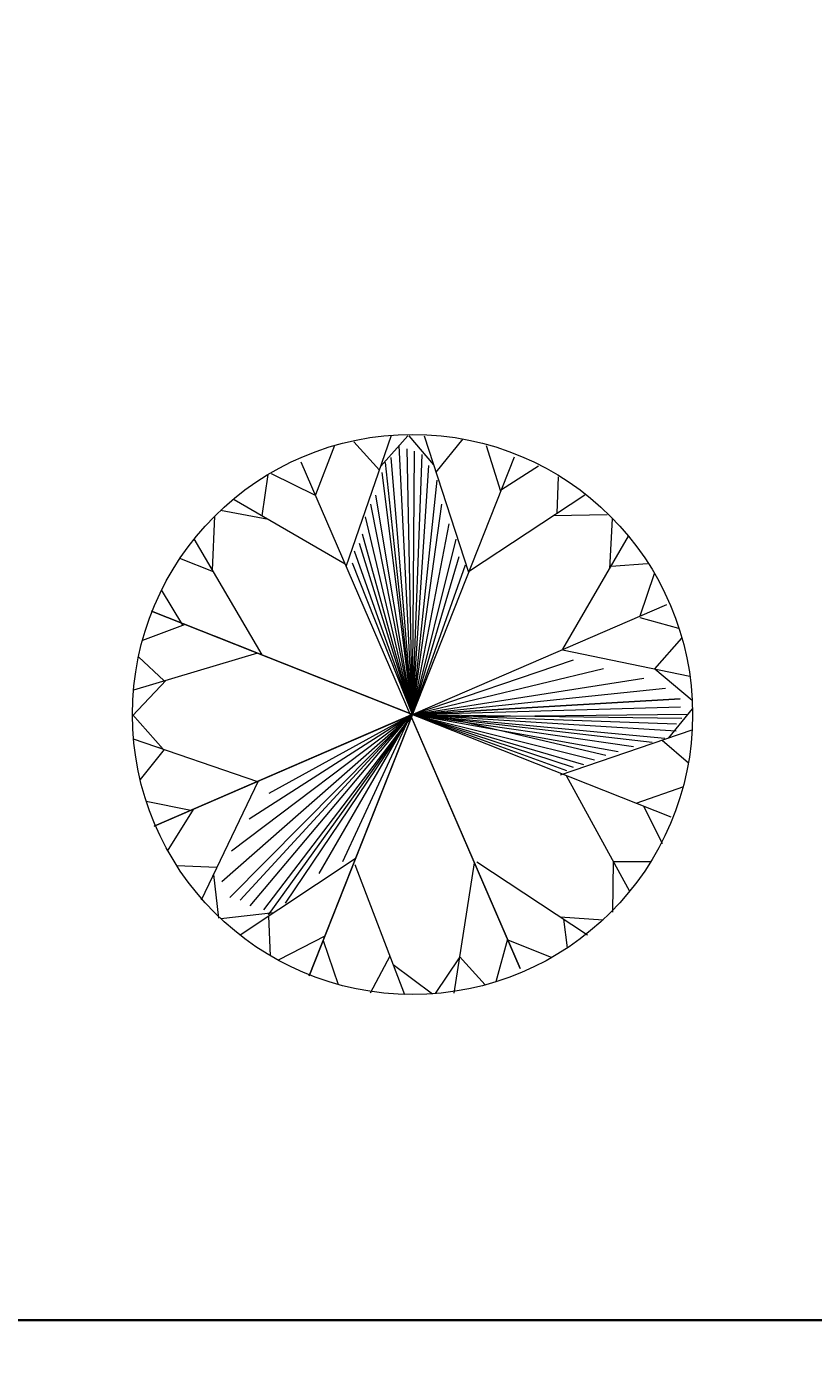
# Model space of a CAD drawing. Units: inches. Extents: x 8049 to 8459, y 820 to 1350.
# Tile 10 of 25: x 8157 to 8170, y 853 to 877. Entities that reach past the tile are written whole.
import ezdxf

# ---------------------------------------------------------------- set-up
doc = ezdxf.new("R2010")
doc.units = ezdxf.units.IN
doc.header["$MEASUREMENT"] = 0
for name, color, linetype, lineweight in [('A-ANNO-DIMS', 2, 'Continuous', 18), ('C-SITE-WALL', 7, 'Continuous', 35), ('zelen', 69, 'Continuous', 13)]:
    doc.layers.add(name, color=color, linetype=linetype, lineweight=lineweight)
doc.styles.get("Standard").update_dxf_attribs({"font": 'arial.ttf'})
doc.dimstyles.get("Standard").update_dxf_attribs({"dimtxt": 0.18, "dimasz": 0.18, "dimexe": 0.18, "dimexo": 0.0625, "dimgap": 0.09, "dimtad": 0, "dimtih": 1, "dimtoh": 1, "dimdec": 4, "dimzin": 0, "dimdsep": 46, "dimtxsty": 'Standard', "dimcen": 0.09, "dimadec": 0, "dimazin": 0, "dimtfac": 1, "dimtdec": 4, "dimtofl": 0, "dimtmove": 0, "dimatfit": 3, "dimfxl": 1, "dimtolj": 1, "dimtzin": 0, "dimarcsym": 0})

# ---------------------------------------------------------------- blocks, each defined once
blk = doc.blocks.new('T40C')
for p, q in [((-0.1219, 0.4263), (-0.1133, 0.5002)), ((-0.0016, 0.4444), (-0.055, 0.5069)), ((-0.0016, 0.0138), (-0.0016, 0.5115)), ((-0.0016, 0.5115), (-0.0016, -0.4769)), ((-0.0016, 0.4364), (0.0585, 0.5048)), ((0.1041, 0.4402), (0.0754, 0.5038)), ((-0.0047, 0.2984), (-0.1711, 0.4799)), ((-0.0016, 0.2889), (0.1386, 0.4896)), ((0.2217, 0.4068), (0.1848, 0.4759)), ((-0.2374, 0.3843), (-0.221, 0.4586)), ((-0.1327, 0.438), (-0.2166, 0.4607)), ((0.0979, 0.4313), (0.1806, 0.4751)), ((0.2091, 0.2244), (0.2252, 0.4573)), ((-0.2, 0.2178), (-0.2513, 0.4459)), ((-0.0016, 0.0138), (0.1054, 0.4378)), ((-0.0016, 0.0138), (0.1166, 0.4328)), ((0.0011, 0.0164), (0.1417, 0.4349)), ((0.0011, 0.0164), (0.1801, 0.4343)), ((0.0011, 0.0164), (0.161, 0.432)), ((-0.2369, 0.3817), (-0.2976, 0.4118)), ((-0.0016, 0.0138), (0.2033, 0.4135)), ((-0.0016, 0.0138), (0.0852, 0.4075)), ((0.2208, 0.3933), (0.2879, 0.4166)), ((-0.3045, 0.3219), (-0.313, 0.3998)), ((0.2979, 0.3132), (0.3134, 0.399)), ((0.3508, 0.3661), (-0.3487, -0.3333)), ((0.0011, 0.0164), (-0.3443, 0.3618)), ((-0.3443, 0.3618), (0.3464, -0.329)), ((-0.0016, 0.0138), (0.2072, 0.3567)), ((0.0011, 0.0164), (0.3508, 0.3661)), ((0.0011, 0.0164), (0.0491, 0.3369)), ((-0.3055, 0.3229), (-0.3893, 0.3231)), ((0.3008, 0.3162), (0.3801, 0.3306)), ((-0.3838, 0.2523), (-0.4084, 0.2975)), ((-0.0016, 0.0138), (0.1989, 0.2926)), ((0.0011, 0.0164), (0.0175, 0.3021)), ((0.3847, 0.2335), (0.4047, 0.2984)), ((-0.2034, 0.2144), (-0.4335, 0.2627)), ((-0.377, 0.2509), (-0.4492, 0.2275)), ((-0.0016, 0.0138), (0.1836, 0.2378)), ((0.2092, 0.2254), (0.4418, 0.2362)), ((0.3861, 0.2336), (0.4597, 0.1963)), ((0.3915, 0.2339), (0.3982, 0.2342)), ((-0.4278, 0.1246), (-0.4601, 0.209)), ((0.4263, 0.1181), (0.4586, 0.1989)), ((-0.2946, 0.0138), (-0.4744, 0.1635)), ((0.2937, 0.0138), (0.4738, 0.1555)), ((-0.4281, 0.1249), (-0.4899, 0.1006)), ((0.4291, 0.1204), (0.4873, 0.0978)), ((-0.4418, 0.0138), (-0.4967, 0.0634)), ((0.4315, 0.0138), (0.491, 0.0679)), ((-0.4277, 0.0138), (-0.4952, -0.0443)), ((0.4953, 0.0138), (-0.4939, 0.0138)), ((-0.2846, 0.0167), (-0.4721, -0.1432)), ((-0.0016, 0.0138), (-0.4477, -0.1559)), ((-0.0016, 0.0138), (-0.4464, -0.1312)), ((-0.0016, 0.0138), (-0.4422, -0.1429)), ((-0.0016, 0.0138), (-0.4379, -0.1735)), ((-0.0016, 0.0138), (-0.4328, -0.1117)), ((-0.0016, 0.0138), (-0.4324, -0.1862)), ((-0.4324, -0.1862), (-0.0016, 0.0138)), ((-0.0016, 0.0138), (-0.4146, -0.0968)), ((-0.0016, 0.0138), (-0.4013, -0.1946)), ((-0.0016, 0.0138), (-0.3864, -0.0775)), ((-0.0016, 0.0138), (-0.3647, -0.0593)), ((-0.0016, 0.0138), (-0.3588, -0.1967)), ((-0.0016, 0.0138), (-0.3309, -0.0302)), ((-0.0016, 0.0138), (-0.3156, -0.0151)), ((-0.0016, 0.0138), (-0.3007, -0.0042)), ((-0.0016, 0.0138), (-0.2917, 0.0059)), ((-0.0016, 0.0138), (-0.2861, -0.1863)), ((-0.0016, 0.0138), (-0.2311, -0.181)), ((-0.0016, 0.0138), (-0.0528, -0.0021)), ((-0.0016, 0.0138), (-0.0528, -0.0021)), ((-0.0016, 0.0138), (0.0011, 0.0164)), ((-0.0016, 0.0138), (0.4953, 0.0138)), ((-0.0016, 0.0138), (0.0088, -0.2669)), ((-0.0016, 0.0138), (0.0243, -0.2768)), ((-0.0016, 0.0138), (0.0408, -0.3033)), ((-0.0016, 0.0138), (0.0625, -0.3241)), ((-0.0016, 0.0138), (0.0872, -0.3518)), ((-0.0016, 0.0138), (0.1104, -0.3878)), ((-0.0016, 0.0138), (0.1339, -0.4064)), ((-0.0016, 0.0138), (0.1521, -0.4202)), ((-0.0016, 0.0138), (0.1669, -0.4211)), ((-0.0016, 0.0138), (0.1801, -0.4202)), ((-0.0016, 0.0138), (0.1959, -0.4202)), ((-0.0016, 0.0138), (0.2013, -0.3955)), ((-0.0016, 0.0138), (0.2072, -0.3832)), ((-0.0016, 0.0138), (0.2062, -0.3647)), ((-0.0016, 0.0138), (0.2018, -0.3233)), ((-0.0016, 0.0138), (0.2038, -0.3052)), ((-0.0016, 0.0138), (0.2044, -0.2809)), ((-0.0016, 0.0138), (0.1983, -0.2504)), ((-0.0016, 0.0138), (0.197, -0.2334)), ((-0.0016, 0.0138), (0.2007, -0.2173)), ((-0.0016, 0.0138), (0.1959, -0.1959)), ((0.285, 0.0138), (0.4722, -0.133)), ((0.2917, 0.0138), (0.3747, 0.0138)), ((0.4349, 0.0169), (0.4927, -0.0276)), ((-0.0528, -0.0021), (-0.4551, -0.1664)), ((-0.0528, -0.0021), (-0.3463, -0.045)), ((-0.4294, -0.1068), (-0.4874, -0.0863)), ((0.4191, -0.0914), (0.4833, -0.0909)), ((0.4217, -0.0934), (0.4533, -0.184)), ((-0.4387, -0.1147), (-0.459, -0.1779)), ((0.2042, -0.1867), (0.2149, -0.4325)), ((0.2071, -0.1897), (0.4318, -0.2236)), ((-0.3712, -0.2192), (-0.4529, -0.1923)), ((-0.2066, -0.1906), (-0.4335, -0.23)), ((-0.2067, -0.1914), (-0.2414, -0.4204)), ((0.3628, -0.2132), (0.4476, -0.1967)), ((-0.3712, -0.2192), (-0.3953, -0.2872)), ((0.3755, -0.2151), (0.3928, -0.2871)), ((-0.0016, -0.2596), (-0.1424, -0.4599)), ((-0.0016, -0.2565), (0.16, -0.4525)), ((0.3007, -0.2833), (0.3874, -0.2905)), ((0.3008, -0.2851), (0.3017, -0.3787)), ((-0.3126, -0.2938), (-0.3837, -0.3016)), ((-0.3124, -0.2971), (-0.3082, -0.3761)), ((-0.2315, -0.3548), (-0.2033, -0.4394)), ((-0.2322, -0.3601), (-0.2902, -0.3882)), ((0.2123, -0.3741), (0.1875, -0.442)), ((0.212, -0.3667), (0.2724, -0.3967)), ((0.1172, -0.4006), (0.0947, -0.4728)), ((-0.1046, -0.4061), (-0.1917, -0.4425)), ((-0.1086, -0.4118), (-0.0869, -0.4727)), ((-0.0016, -0.4144), (-0.047, -0.4779)), ((-0.0016, -0.4109), (0.0515, -0.477)), ((0.1259, -0.4112), (0.1857, -0.4428))]:
    blk.add_line(p, q)
blk.add_circle((-0.0016, 0.0138), 0.496)
blk = doc.blocks.new('*D58')
at = {"layer": 'A-ANNO-DIMS', "color": 0, "lineweight": -2, "transparency": 16777216}
for p, q in [((8139.397, 1162.808), (8139.397, 820.091)), ((8175.397, 1162.808), (8175.397, 820.091)), ((8139.577, 820.271), (8157.179, 820.271)), ((8175.217, 820.271), (8157.616, 820.271))]:
    blk.add_line(p, q, dxfattribs=at)
at = {"layer": 'A-ANNO-DIMS', "color": 0, "transparency": 16777216}
for points in [[(8139.577, 820.301), (8139.577, 820.241), (8139.397, 820.271)], [(8175.217, 820.301), (8175.217, 820.241), (8175.397, 820.271)]]:
    blk.add_solid(points, dxfattribs=at)
at = {"layer": 'Defpoints', "color": 0, "transparency": 16777216}
for p in [(8139.397, 1162.871), (8175.397, 1162.871), (8175.397, 820.271)]:
    blk.add_point(p, dxfattribs=at)
at = {"layer": 'A-ANNO-DIMS', "color": 0, "transparency": 16777216, "insert": (8157.397, 820.271), "char_height": 0.18, "attachment_point": 5}
blk.add_mtext('\\A1;36', dxfattribs=at)
blk = doc.blocks.new('*D76')
at = {"layer": 'A-ANNO-DIMS', "color": 0, "lineweight": -2, "transparency": 16777216}
for p, q in [((8083.397, 1054.808), (8083.397, 820.091)), ((8299.397, 1054.808), (8299.397, 820.091)), ((8083.577, 820.271), (8191.107, 820.271)), ((8299.217, 820.271), (8191.688, 820.271))]:
    blk.add_line(p, q, dxfattribs=at)
at = {"layer": 'A-ANNO-DIMS', "color": 0, "transparency": 16777216}
for points in [[(8083.577, 820.301), (8083.577, 820.241), (8083.397, 820.271)], [(8299.217, 820.301), (8299.217, 820.241), (8299.397, 820.271)]]:
    blk.add_solid(points, dxfattribs=at)
at = {"layer": 'Defpoints', "color": 0, "transparency": 16777216}
for p in [(8083.397, 1054.871), (8299.397, 1054.871), (8299.397, 820.271)]:
    blk.add_point(p, dxfattribs=at)
at = {"layer": 'A-ANNO-DIMS', "color": 0, "transparency": 16777216, "insert": (8191.397, 820.271), "char_height": 0.18, "attachment_point": 5}
blk.add_mtext('\\A1;216', dxfattribs=at)

msp = doc.modelspace()

# ---------------------------------------------------------------- linework, layer by layer
at = {"layer": 'C-SITE-WALL'}
msp.add_line((8083.3974, 853.8706), (8219.8974, 853.8706), dxfattribs=at)

# ---------------------------------------------------------------- block references
at = {"layer": 'zelen', "xscale": 9.920223989974332, "yscale": 9.920223989974332, "zscale": 9.920223989974332, "rotation": 158.4000000000004}
msp.add_blockref('T40C', (8163.4624, 864.644), dxfattribs=at)

# ---------------------------------------------------------------- dimensions: what is measured, and where the dimension line sits
at = {"layer": 'A-ANNO-DIMS'}
for base, p1, p2, picture, middle in [((8175.3974, 820.2706), (8139.3974, 1162.8706), (8175.3974, 1162.8706), '*D58', (8157.3974, 820.2706)), ((8299.3974, 820.2706), (8083.3974, 1054.8706), (8299.3974, 1054.8706), '*D76', (8191.3974, 820.2706))]:
    dim = msp.add_linear_dim(base=base, p1=p1, p2=p2, dimstyle='Standard', override={"dimdec": 0, "dimlfac": 1, "dimrnd": 0, "dimzin": 0, "dimdsep": 46, "dimlunit": 2}, dxfattribs=at)
    dim.commit()
    dim.dimension.update_dxf_attribs({"geometry": picture, "text_midpoint": middle})

doc.saveas('drawing.dxf')
